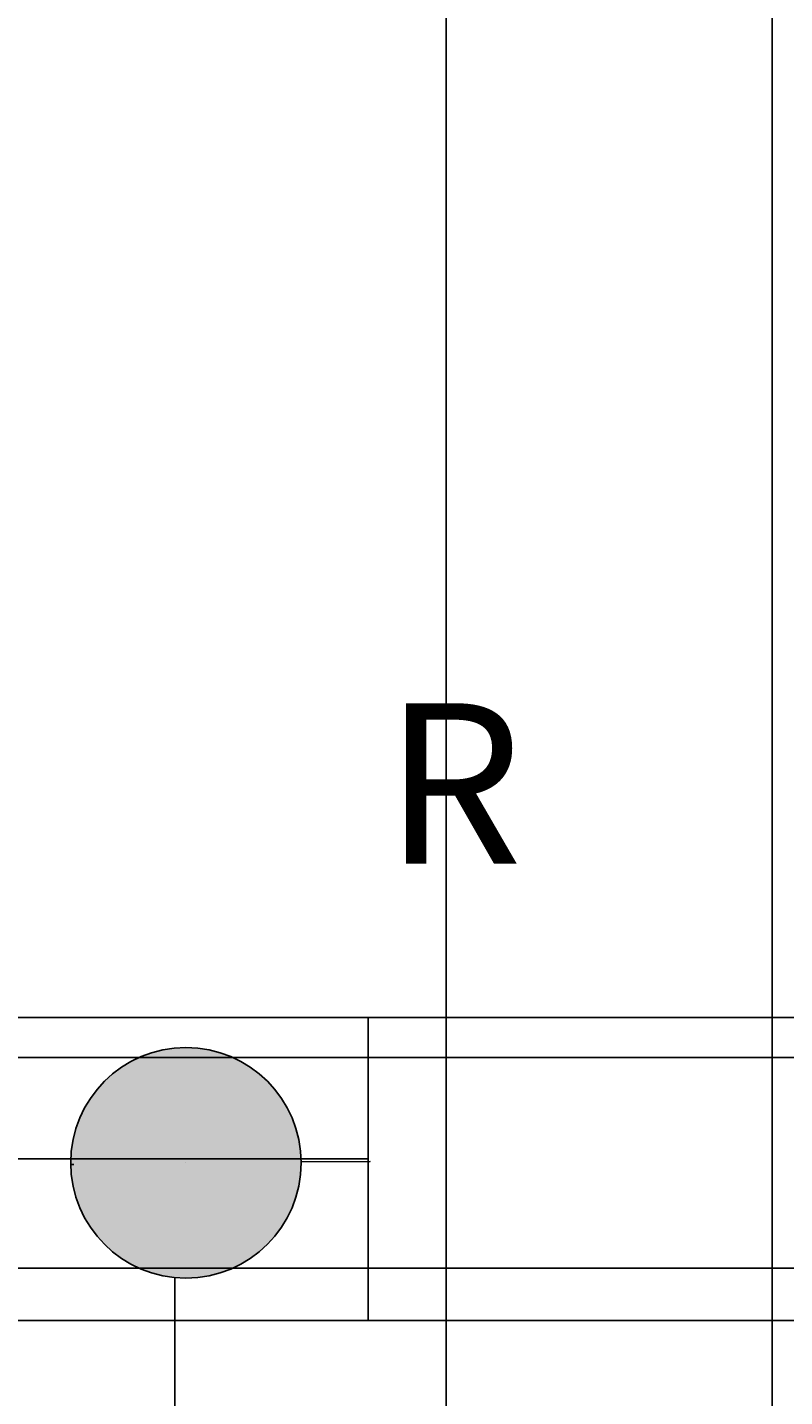
# Model space of a CAD drawing. Units: inches. Extents: x 35362 to 73946, y 43607 to 67532.
# Tile 125 of 134: x 51337 to 52380, y 48793 to 50677. Entities that reach past the tile are written whole.
import ezdxf

# ---------------------------------------------------------------- set-up
doc = ezdxf.new("R2010")
doc.units = ezdxf.units.IN
doc.header["$MEASUREMENT"] = 0
for name, color, linetype, lineweight in [('A-ANNO-DIMS', 2, 'Continuous', 18), ('E-ANNO-TEXT', 5, 'Continuous', 18), ('E-SYMB', 1, 'Continuous', 25), ('E-SYMB-PATT', 1, 'Continuous', 13), ('E-WIRE', 3, 'Continuous', 25)]:
    doc.layers.add(name, color=color, linetype=linetype, lineweight=lineweight)
doc.styles.get("Standard").update_dxf_attribs({"font": 'arial.ttf'})
doc.dimstyles.get("Standard").update_dxf_attribs({"dimtxt": 0.18, "dimasz": 0.18, "dimexe": 0.18, "dimexo": 0.0625, "dimgap": 0.09, "dimtad": 0, "dimtih": 1, "dimtoh": 1, "dimdec": 4, "dimzin": 0, "dimdsep": 46, "dimtxsty": 'Standard', "dimcen": 0.09, "dimadec": 0, "dimazin": 0, "dimtfac": 1, "dimtdec": 4, "dimtofl": 0, "dimtmove": 0, "dimatfit": 3, "dimfxl": 1, "dimtolj": 1, "dimtzin": 0, "dimarcsym": 0})

# ---------------------------------------------------------------- blocks, each defined once
blk = doc.blocks.new('*D11')
at = {"layer": 'A-ANNO-DIMS', "color": 0, "lineweight": -2, "transparency": 16777216}
for p, q in [((47978.7, 56028.8), (47978.7, 43606.7)), ((53109.8, 56028.8), (53109.8, 43606.7)), ((47978.8, 43606.9), (50543.9, 43606.9)), ((53109.6, 43606.9), (50544.6, 43606.9))]:
    blk.add_line(p, q, dxfattribs=at)
at = {"layer": 'A-ANNO-DIMS', "color": 0, "transparency": 16777216}
for points in [[(47978.8, 43606.9), (47978.8, 43606.8), (47978.7, 43606.9)], [(53109.6, 43606.9), (53109.6, 43606.8), (53109.8, 43606.9)]]:
    blk.add_solid(points, dxfattribs=at)
at = {"layer": 'Defpoints', "color": 0, "transparency": 16777216}
for p in [(47978.7, 56028.8), (53109.8, 56028.8), (53109.8, 43606.9)]:
    blk.add_point(p, dxfattribs=at)
at = {"layer": 'A-ANNO-DIMS', "color": 0, "transparency": 16777216, "insert": (50544.2, 43606.9), "char_height": 0.18, "attachment_point": 5}
blk.add_mtext('\\A1;5131', dxfattribs=at)
blk = doc.blocks.new('*D17')
at = {"layer": 'A-ANNO-DIMS', "color": 0, "lineweight": -2, "transparency": 16777216}
for p, q in [((49923.3, 61293.2), (49923.3, 43606.7)), ((51913.9, 61293.2), (51913.9, 43606.7)), ((49923.5, 43606.9), (50918.2, 43606.9)), ((51913.8, 43606.9), (50919.1, 43606.9))]:
    blk.add_line(p, q, dxfattribs=at)
at = {"layer": 'A-ANNO-DIMS', "color": 0, "transparency": 16777216}
for points in [[(49923.5, 43606.9), (49923.5, 43606.8), (49923.3, 43606.9)], [(51913.8, 43606.9), (51913.8, 43606.8), (51913.9, 43606.9)]]:
    blk.add_solid(points, dxfattribs=at)
at = {"layer": 'Defpoints', "color": 0, "transparency": 16777216}
for p in [(49923.3, 61293.3), (51913.9, 61293.3), (51913.9, 43606.9)]:
    blk.add_point(p, dxfattribs=at)
at = {"layer": 'A-ANNO-DIMS', "color": 0, "transparency": 16777216, "insert": (50918.6, 43606.9), "char_height": 0.18, "attachment_point": 5}
blk.add_mtext('\\A1;1990.6', dxfattribs=at)
blk = doc.blocks.new('*D40')
at = {"layer": 'A-ANNO-DIMS', "color": 0, "lineweight": -2, "transparency": 16777216}
for p, q in [((56873.5, 53351.5), (35361.8, 53351.5)), ((35361.9, 53351.3), (35361.9, 51333.3)), ((35361.9, 49314.8), (35361.9, 51332.9)), ((51806.5, 49314.7), (35361.8, 49314.7))]:
    blk.add_line(p, q, dxfattribs=at)
at = {"layer": 'A-ANNO-DIMS', "color": 0, "transparency": 16777216}
for points in [[(35361.9, 53351.3), (35362, 53351.3), (35361.9, 53351.5)], [(35361.9, 49314.8), (35362, 49314.8), (35361.9, 49314.7)]]:
    blk.add_solid(points, dxfattribs=at)
at = {"layer": 'Defpoints', "color": 0, "transparency": 16777216}
for p in [(35361.9, 53351.5), (56873.6, 53351.5), (51806.5, 49314.7)]:
    blk.add_point(p, dxfattribs=at)
at = {"layer": 'A-ANNO-DIMS', "color": 0, "transparency": 16777216, "insert": (35361.9, 51333.1), "char_height": 0.18, "attachment_point": 5}
blk.add_mtext('\\A1;4036.9', dxfattribs=at)
blk = doc.blocks.new('*D67')
at = {"layer": 'A-ANNO-DIMS', "color": 0, "lineweight": -2, "transparency": 16777216}
for p, q in [((56873.5, 53351.5), (35361.8, 53351.5)), ((35361.9, 53351.3), (35361.9, 49400.9)), ((35361.9, 45450.1), (35361.9, 49400.5)), ((53793.6, 45449.9), (35361.8, 45449.9))]:
    blk.add_line(p, q, dxfattribs=at)
at = {"layer": 'A-ANNO-DIMS', "color": 0, "transparency": 16777216}
for points in [[(35361.9, 53351.3), (35362, 53351.3), (35361.9, 53351.5)], [(35361.9, 45450.1), (35362, 45450.1), (35361.9, 45449.9)]]:
    blk.add_solid(points, dxfattribs=at)
at = {"layer": 'Defpoints', "color": 0, "transparency": 16777216}
for p in [(35361.9, 53351.5), (56873.6, 53351.5), (53793.6, 45449.9)]:
    blk.add_point(p, dxfattribs=at)
at = {"layer": 'A-ANNO-DIMS', "color": 0, "transparency": 16777216, "insert": (35361.9, 49400.7), "char_height": 0.18, "attachment_point": 5}
blk.add_mtext('\\A1;7901.6', dxfattribs=at)
blk = doc.blocks.new('*D84')
at = {"layer": 'A-ANNO-DIMS', "color": 0, "lineweight": -2, "transparency": 16777216}
for p, q in [((55540.2, 49259.9), (35361.8, 49259.9)), ((35361.9, 49259.8), (35361.9, 49115.1)), ((35361.9, 48970.2), (35361.9, 49114.8)), ((55540.2, 48970), (35361.8, 48970))]:
    blk.add_line(p, q, dxfattribs=at)
at = {"layer": 'A-ANNO-DIMS', "color": 0, "transparency": 16777216}
for points in [[(35361.9, 49259.8), (35362, 49259.8), (35361.9, 49259.9)], [(35361.9, 48970.2), (35362, 48970.2), (35361.9, 48970)]]:
    blk.add_solid(points, dxfattribs=at)
at = {"layer": 'Defpoints', "color": 0, "transparency": 16777216}
for p in [(35361.9, 49259.9), (55540.3, 49259.9), (55540.3, 48970)]:
    blk.add_point(p, dxfattribs=at)
at = {"layer": 'A-ANNO-DIMS', "color": 0, "transparency": 16777216, "insert": (35361.9, 49115), "char_height": 0.18, "attachment_point": 5}
blk.add_mtext('\\A1;289.96', dxfattribs=at)
blk = doc.blocks.new('*D88')
at = {"layer": 'A-ANNO-DIMS', "color": 0, "lineweight": -2, "transparency": 16777216}
for p, q in [((52362.6, 48318.3), (52362.6, 67531.7)), ((52362.7, 67531.5), (52432.1, 67531.5)), ((52502.2, 67531.5), (52432.8, 67531.5)), ((52502.4, 48318.3), (52502.4, 67531.7))]:
    blk.add_line(p, q, dxfattribs=at)
at = {"layer": 'A-ANNO-DIMS', "color": 0, "transparency": 16777216}
for points in [[(52362.7, 67531.5), (52362.7, 67531.5), (52362.6, 67531.5)], [(52502.2, 67531.5), (52502.2, 67531.5), (52502.4, 67531.5)]]:
    blk.add_solid(points, dxfattribs=at)
at = {"layer": 'Defpoints', "color": 0, "transparency": 16777216}
for p in [(52502.4, 67531.5), (52362.6, 48318.3), (52502.4, 48318.3)]:
    blk.add_point(p, dxfattribs=at)
at = {"layer": 'A-ANNO-DIMS', "color": 0, "transparency": 16777216, "insert": (52432.5, 67531.5), "char_height": 0.18, "attachment_point": 5}
blk.add_mtext('\\A1;139.8', dxfattribs=at)
blk = doc.blocks.new('*D89')
at = {"layer": 'A-ANNO-DIMS', "color": 0, "lineweight": -2, "transparency": 16777216}
for p, q in [((53707.7, 48897.7), (35361.8, 48897.7)), ((35361.9, 48897.6), (35361.9, 48303.2)), ((35361.9, 47708.4), (35361.9, 48302.8)), ((53707.7, 47708.2), (35361.8, 47708.2))]:
    blk.add_line(p, q, dxfattribs=at)
at = {"layer": 'A-ANNO-DIMS', "color": 0, "transparency": 16777216}
for points in [[(35361.9, 48897.6), (35362, 48897.6), (35361.9, 48897.7)], [(35361.9, 47708.4), (35362, 47708.4), (35361.9, 47708.2)]]:
    blk.add_solid(points, dxfattribs=at)
at = {"layer": 'Defpoints', "color": 0, "transparency": 16777216}
for p in [(53707.8, 48897.7), (35361.9, 47708.2), (53707.8, 47708.2)]:
    blk.add_point(p, dxfattribs=at)
at = {"layer": 'A-ANNO-DIMS', "color": 0, "transparency": 16777216, "insert": (35361.9, 48303), "char_height": 0.18, "attachment_point": 5}
blk.add_mtext('\\A1;1189.5', dxfattribs=at)
blk = doc.blocks.new('*D117')
at = {"layer": 'A-ANNO-DIMS', "color": 0, "lineweight": -2, "transparency": 16777216}
for p, q in [((51555.6, 49114.8), (51555.8, 49114.8)), ((51555.7, 49114.7), (51555.7, 49114.9)), ((51809.4, 49116.7), (51714.5, 49116))]:
    blk.add_line(p, q, dxfattribs=at)
at = {"layer": 'A-ANNO-DIMS', "color": 0, "transparency": 16777216}
blk.add_solid([(51714.5, 49116), (51714.5, 49116), (51714.3, 49116)], dxfattribs=at)
at = {"layer": 'Defpoints', "color": 0, "transparency": 16777216}
for p in [(51397.1, 49113.6), (51714.3, 49116)]:
    blk.add_point(p, dxfattribs=at)
at = {"layer": 'A-ANNO-DIMS', "color": 0, "transparency": 16777216, "insert": (51809.9, 49116.7), "char_height": 0.18, "attachment_point": 5}
blk.add_mtext('\\A1;∅317.2', dxfattribs=at)

msp = doc.modelspace()

# ---------------------------------------------------------------- hatches: boundary and pattern name
at = {"layer": 'E-SYMB-PATT'}
h = msp.add_hatch(color=256, dxfattribs=at)
h.dxf.hatch_style = 1
h.paths.add_polyline_path([(51714.267, 49112.547, 0.41839319), (51555.678, 49273.413, 0.41839319), (51397.088, 49112.547)])
h.paths.add_polyline_path([(51714.267, 49112.547), (51397.088, 49112.547, 0.41004625), (51555.678, 48956.201, 0.41004625)])

# ---------------------------------------------------------------- linework, layer by layer
at = {"layer": 'E-SYMB'}
for p, q in [((51714.196, 49120.079), (51285.595, 49120.079)), ((51714.266, 49117.122), (51713.58, 49117.122)), ((51806.517, 49120.079), (51714.196, 49120.079)), ((51401.559, 49112.547), (51397.088, 49112.547))]:
    msp.add_line(p, q, dxfattribs=at)
msp.add_lwpolyline([(52563.135, 49314.669), (52563.135, 48897.738), (51806.517, 48897.738), (51806.517, 49314.669)], close=True, dxfattribs=at)
msp.add_circle((51555.678, 49114.807), 158.606, dxfattribs=at)
at = {"layer": 'E-WIRE'}
msp.add_line((51540.551, 48956.924), (51540.551, 47918.089), dxfattribs=at)

# ---------------------------------------------------------------- texts
at = {"layer": 'E-ANNO-TEXT'}
msp.add_text('R', height=220.866, dxfattribs=at).set_placement((51828.295, 49526.315))

# ---------------------------------------------------------------- dimensions: what is measured, and where the dimension line sits
at = {"layer": 'A-ANNO-DIMS'}
for base, p1, p2, override, picture, middle in [((52502.363, 67531.512), (52362.557, 48318.269), (52502.363, 48318.269), {"dimdec": 1, "dimlfac": 1, "dimrnd": 0, "dimzin": 0, "dimdsep": 46, "dimlunit": 2}, '*D88', (52432.46, 67531.512)), ((51913.931, 43606.859), (49923.307, 61293.286), (51913.931, 61293.286), {"dimdec": 1, "dimlfac": 1, "dimrnd": 0, "dimzin": 0, "dimdsep": 46, "dimlunit": 2}, '*D17', (50918.619, 43606.859)), ((53109.76, 43606.859), (47978.665, 56028.836), (53109.76, 56028.836), {"dimdec": 0, "dimlfac": 1, "dimrnd": 0, "dimzin": 0, "dimdsep": 46, "dimlunit": 2}, '*D11', (50544.212, 43606.859))]:
    dim = msp.add_linear_dim(base=base, p1=p1, p2=p2, dimstyle='Standard', override=override, dxfattribs=at)
    dim.commit()
    dim.dimension.update_dxf_attribs({"geometry": picture, "text_midpoint": middle})
for base, p1, p2, override, picture, middle in [((35361.949, 53351.529), (51806.517, 49314.669), (56873.602, 53351.529), {"dimdec": 1, "dimlfac": 1, "dimrnd": 0, "dimzin": 0, "dimdsep": 46, "dimlunit": 2}, '*D40', (35361.949, 51333.099)), ((35361.949, 53351.529), (53793.638, 45449.894), (56873.602, 53351.529), {"dimdec": 1, "dimlfac": 1, "dimrnd": 0, "dimzin": 0, "dimdsep": 46, "dimlunit": 2}, '*D67', (35361.949, 49400.712)), ((35361.9491, 49259.9353), (55540.2972, 48969.9796), (55540.2972, 49259.9353), {"dimdec": 2, "dimlfac": 1, "dimrnd": 0, "dimzin": 0, "dimdsep": 46, "dimlunit": 2}, '*D84', (35361.9491, 49114.9575)), ((35361.949, 47708.216), (53707.781, 48897.738), (53707.781, 47708.216), {"dimdec": 1, "dimlfac": 1, "dimrnd": 0, "dimzin": 0, "dimdsep": 46, "dimlunit": 2}, '*D89', (35361.949, 48302.977))]:
    dim = msp.add_linear_dim(base=base, p1=p1, p2=p2, angle=90, dimstyle='Standard', override=override, dxfattribs=at)
    dim.commit()
    dim.dimension.update_dxf_attribs({"geometry": picture, "text_midpoint": middle})
dim = msp.add_diameter_dim_2p(p1=(51397.076, 49113.611), p2=(51714.279, 49116.002), dimstyle='Standard', override={"dimdec": 1, "dimlfac": 1, "dimrnd": 0, "dimzin": 0, "dimdsep": 46, "dimlunit": 2}, dxfattribs=at)
dim.commit()
dim.dimension.update_dxf_attribs({"geometry": '*D117', "text_midpoint": (51809.44, 49116.719), "dimtype": 163})

doc.saveas('drawing.dxf')
